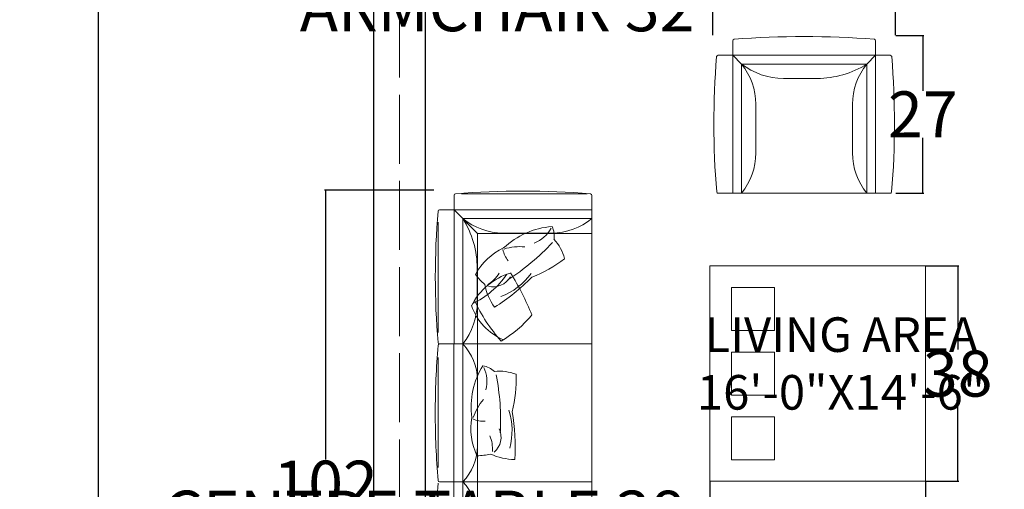
# Model space of a CAD drawing. Units: inches. Extents: x -48 to 50072, y 0 to 21068.
# Tile 49 of 75: x -48 to 123, y 738 to 819. Entities that reach past the tile are written whole.
import ezdxf

# ---------------------------------------------------------------- set-up
doc = ezdxf.new("R2010")
doc.units = ezdxf.units.IN
doc.header["$MEASUREMENT"] = 0
doc.linetypes.add('ACAD_ISO02W100', pattern=[15, 12, -3])
for name, color, linetype, lineweight in [('A-ANNO-DIMS', 2, 'Continuous', 18), ('A-AREA-IDEN', 7, 'Continuous', 18), ('C-PROP', 7, 'Continuous', 25), ('C-PROP-REF', 32, 'ACAD_ISO02W100', 13), ('FURNITURE', 44, 'Continuous', 18)]:
    doc.layers.add(name, color=color, linetype=linetype, lineweight=lineweight)
doc.styles.get("Standard").update_dxf_attribs({"font": 'arial.ttf'})
doc.dimstyles.get("Standard").update_dxf_attribs({"dimtxt": 8, "dimasz": 0.18, "dimexe": 0.18, "dimexo": 0.0625, "dimgap": 0.09, "dimtad": 0, "dimtih": 1, "dimtoh": 1, "dimdec": 1, "dimzin": 0, "dimdsep": 46, "dimlunit": 4, "dimtxsty": 'Standard', "dimblk": 'ARCHTICK', "dimcen": 0.09, "dimadec": 0, "dimazin": 0, "dimtfac": 1, "dimtdec": 1, "dimtofl": 0, "dimtmove": 0, "dimatfit": 3, "dimldrblk": 'ARCHTICK', "dimfxl": 1, "dimtolj": 1, "dimtzin": 0, "dimarcsym": 0})

# ---------------------------------------------------------------- blocks, each defined once
blk = doc.blocks.new('CENTER TABLE')
at = {"layer": 'FURNITURE'}
for points in [[(7434.06, 1871.2), (7464.06, 1871.2), (7464.06, 1901.2), (7434.06, 1901.2)], [(7455.06, 1898.2), (7461.06, 1898.2), (7461.06, 1892.2), (7455.06, 1892.2)], [(7455.06, 1883.2), (7461.06, 1883.2), (7461.06, 1889.2), (7455.06, 1889.2)], [(7455.06, 1874.2), (7461.06, 1874.2), (7461.06, 1880.2), (7455.06, 1880.2)]]:
    blk.add_lwpolyline(points, close=True, dxfattribs=at)
blk = doc.blocks.new('WRG')
at = {"layer": 'FURNITURE'}
for centre, radius, start, end in [((-5881.03, 869.32), 50.97, 111.3371, 122.4176), ((-5914.7, 898.39), 23.82, 30.3068, 50.5663), ((-5895.33, 916.33), 13.61, 197.0126, 242.9429), ((-5918.49, 896.36), 18.43, 25.9005, 55.6513), ((-5905.57, 915.66), 12.15, 289.4501, 336.7699), ((-5915.78, 934.22), 32.17, 294.0815, 312.2768)]:
    blk.add_arc(centre, radius, start, end, dxfattribs=at)
blk = doc.blocks.new('DFGS')
at = {"layer": 'FURNITURE'}
for centre, radius, start, end in [((-6087.14, 813.36), 9.64, 104.9394, 132.5633), ((-6112.38, 805.26), 28.66, 21.6133, 37.4184), ((-6094.33, 816.04), 4.48, 81.3108, 116.3418), ((-6126.91, 783.89), 49.66, 32.8076, 46.9), ((-6080.05, 821.2), 16.31, 184.0297, 223.6176), ((-6099.45, 813.66), 7.12, 22.214, 60.8038), ((-6080.96, 813.35), 11.17, 174.5959, 197.1556), ((-6094.76, 804.41), 13.97, 20.7975, 53.8819), ((-6116.99, 784.16), 44.49, 32.4999, 45.375), ((-6080.21, 815.37), 12.85, 204.9913, 241.6537), ((-6092.61, 815.13), 5.43, 281.6061, 309.1892), ((-6087.9, 807.73), 4.17, 346.5527, 60.4145), ((-6089.91, 803.33), 6.58, 30.5945, 59.6065), ((-6086.56, 817.99), 12.2, 280.9279, 305.5545), ((-6095.16, 815.51), 14.47, 307.7029, 318.9387)]:
    blk.add_arc(centre, radius, start, end, dxfattribs=at)
blk = doc.blocks.new('3+2 seater sofa')
at = {"layer": 'FURNITURE'}
for p, q in [((1464.23, 900.93), (1464.23, 875.06)), ((1465.03, 901.17), (1486.94, 901.17)), ((1488.22, 900.95), (1488.22, 898.4)), ((1488.22, 898.4), (1464.22, 898.4)), ((1488.22, 898.4), (1484.13, 894.31)), ((1490.75, 898.4), (1488.22, 898.4)), ((1488.22, 898.4), (1488.22, 875.06, 0)), ((1486.69, 896.88), (1464.22, 896.88)), ((1486.69, 896.88), (1486.69, 875.06)), ((1490.98, 877.03), (1490.98, 896.27)), ((1484.13, 894.31, 0), (1464.22, 894.31)), ((1471.21, 894.37), (1479.69, 894.37)), ((1484.13, 894.31), (1484.13, 875.06)), ((1484.18, 888.22), (1484.18, 882.36)), ((1490.74, 875.06), (1464.23, 875.06)), ((1484.13, 875.06), (1490.75, 875.06)), ((1486.69, 863.06), (1486.69, 875.06)), ((1488.23, 851.03, 0), (1488.23, 875.06)), ((1490.98, 872.68), (1490.98, 863.06)), ((1484.15, 868.83), (1484.15, 863.06)), ((1484.15, 857.29), (1484.15, 863.06)), ((1484.15, 863.06, 0), (1484.15, 851.06)), ((1486.69, 863.06), (1486.69, 851.06)), ((1490.98, 853.57), (1490.98, 863.06)), ((1490.74, 851.06), (1464.23, 851.06)), ((1484.13, 851.06), (1490.75, 851.06)), ((1486.69, 839.06), (1486.69, 851.06)), ((1488.23, 827.03, 0), (1488.23, 851.06)), ((1490.98, 848.68), (1490.98, 839.06)), ((1484.15, 844.83), (1484.15, 839.06)), ((1484.15, 833.29), (1484.15, 839.06)), ((1484.15, 839.06, 0), (1484.15, 827.06)), ((1486.69, 839.06), (1486.69, 827.06)), ((1490.98, 829.57), (1490.98, 839.06)), ((1366.11, 826.25), (1366.11, 804.34)), ((1366.35, 827.06), (1392.23, 827.06)), ((1368.88, 803.07), (1368.88, 827.07)), ((1370.4, 804.59), (1370.4, 827.07)), ((1392.23, 800.54), (1392.23, 827.06)), ((1392.23, 800.54), (1392.23, 827.06)), ((1416.23, 800.54), (1416.23, 827.06)), ((1440.23, 800.54), (1440.23, 827.06)), ((1464.23, 800.54), (1464.23, 827.06)), ((1490.74, 827.06), (1464.23, 827.06)), ((1484.13, 827.06), (1490.75, 827.06)), ((1372.92, 820.07), (1372.92, 811.59)), ((1368.88, 803.07), (1372.97, 807.16)), ((1372.97, 807.16), (1392.23, 807.16)), ((1379.07, 807.11), (1384.92, 807.11)), ((1392.23, 807.16), (1392.23, 800.53)), ((1392.23, 807.16), (1392.23, 800.53)), ((1398.46, 807.13), (1404.23, 807.13)), ((1410, 807.13), (1404.23, 807.13)), ((1404.23, 807.13, 0), (1416.23, 807.13)), ((1416.23, 807.16), (1416.23, 800.53)), ((1422.46, 807.13), (1428.23, 807.13)), ((1434, 807.13), (1428.23, 807.13)), ((1428.23, 807.13, 0), (1440.23, 807.13)), ((1440.23, 807.16), (1440.23, 800.53)), ((1446.46, 807.13), (1452.23, 807.13)), ((1458, 807.13), (1452.23, 807.13)), ((1452.23, 807.13, 0), (1464.23, 807.13)), ((1464.23, 807.16), (1464.23, 800.53)), ((1370.4, 804.59), (1392.23, 804.59)), ((1404.23, 804.59), (1392.23, 804.59)), ((1404.23, 804.59), (1416.23, 804.59)), ((1428.23, 804.59), (1416.23, 804.59)), ((1428.23, 804.59), (1440.23, 804.59)), ((1452.23, 804.59), (1440.23, 804.59)), ((1452.23, 804.59), (1464.23, 804.59)), ((1366.33, 803.07), (1368.88, 803.07)), ((1368.88, 800.53), (1368.88, 803.07)), ((1368.88, 803.07), (1392.23, 803.07, 0)), ((1416.26, 803.06, 0), (1392.23, 803.06)), ((1440.26, 803.06, 0), (1416.23, 803.06)), ((1464.26, 803.06, 0), (1440.23, 803.06)), ((1390.25, 800.3), (1371.02, 800.3)), ((1394.6, 800.3), (1404.23, 800.3)), ((1413.72, 800.3), (1404.23, 800.3)), ((1418.6, 800.3), (1428.23, 800.3)), ((1437.72, 800.3), (1428.23, 800.3)), ((1442.6, 800.3), (1452.23, 800.3)), ((1461.72, 800.3), (1452.23, 800.3))]:
    blk.add_line(p, q, dxfattribs=at)
at = {"layer": 'FURNITURE', "ltscale": 3}
for p, q in [((1464.23, 875.06), (1464.23, 851.06)), ((1484.15, 863.06), (1484.15, 875.06)), ((1484.15, 863.06), (1484.15, 851.06)), ((1464.23, 851.06), (1464.23, 827.06)), ((1484.15, 839.06), (1484.15, 851.06)), ((1484.15, 839.06), (1484.15, 827.06)), ((1392.23, 827.06), (1416.23, 827.06)), ((1416.23, 827.06), (1440.23, 827.06)), ((1440.23, 827.06), (1464.23, 827.06)), ((1404.23, 807.13), (1392.23, 807.13)), ((1404.23, 807.13), (1416.23, 807.13)), ((1428.23, 807.13), (1416.23, 807.13)), ((1428.23, 807.13), (1440.23, 807.13)), ((1452.23, 807.13), (1440.23, 807.13)), ((1452.23, 807.13), (1464.23, 807.13))]:
    blk.add_line(p, q, dxfattribs=at)
at = {"layer": 'FURNITURE'}
for centre, radius, start, end in [((1476.31, 758.13), 143.55, 85.3368, 94.7395), ((1464.47, 900.93), 0.255, 94.7915, 180), ((1487.96, 900.95), 0.255, 0, 85.2857), ((1490.75, 898.15), 0.255, 5.7807, 90), ((1354.3, 886.73), 137.18, 355.2142, 4.7858), ((1471.31, 905.62), 11.26, 230.9515, 269.5157), ((1479.6, 905.62), 11.26, 270.4843, 309.0485), ((1500.6, 888.15), 16.42, 147.8787, 179.7559), ((1496.3, 882.45), 12.13, 180.424, 217.563), ((1493.43, 868.68), 9.28, 136.5598, 179.0844), ((1490.74, 874.8), 0.255, 4.5067, 90), ((1490.75, 875.31), 0.255, 270, 354.2193), ((1348.3, 862.96), 143.19, 0.0378, 4.7508), ((1348.3, 863.15), 143.19, 355.2492, 359.9622), ((1493.43, 857.43), 9.28, 180.9156, 223.4402), ((1493.43, 844.68), 9.28, 136.5598, 179.0844), ((1490.74, 851.31), 0.255, 270, 355.4933), ((1348.3, 838.96), 143.19, 0.0378, 4.7508), ((1348.3, 839.15), 143.19, 355.2492, 359.9622), ((1493.43, 833.43), 9.28, 180.9156, 223.4402), ((1509.16, 814.97), 143.55, 175.2605, 184.6632), ((1366.35, 826.81), 0.255, 90, 175.2085), ((1361.66, 819.98), 11.26, 0.4843, 39.0485), ((1490.74, 827.31), 0.255, 270, 355.4933), ((1361.66, 811.68), 11.26, 320.9515, 359.5157), ((1379.14, 790.68), 16.42, 90.2441, 122.1213), ((1384.83, 794.98), 12.13, 52.437, 89.576), ((1398.61, 797.86), 9.28, 90.9156, 133.4402), ((1409.85, 797.86), 9.28, 46.5598, 89.0844), ((1422.61, 797.86), 9.28, 90.9156, 133.4402), ((1433.85, 797.86), 9.28, 46.5598, 89.0844), ((1446.61, 797.86), 9.28, 90.9156, 133.4402), ((1457.85, 797.86), 9.28, 46.5598, 89.0844), ((1366.33, 803.32), 0.255, 184.7143, 270), ((1369.13, 800.53), 0.255, 180, 264.2193), ((1380.55, 936.98), 137.18, 265.2142, 274.7858), ((1391.97, 800.54), 0.255, 274.5067, 0), ((1391.97, 800.53), 0.255, 275.7807, 0), ((1392.48, 800.54), 0.255, 180, 265.4933), ((1392.48, 800.53), 0.255, 180, 264.2193), ((1404.32, 942.98), 143.19, 265.2492, 269.9622), ((1404.13, 942.98), 143.19, 270.0378, 274.7508), ((1415.97, 800.54), 0.255, 274.5067, 0), ((1428.32, 942.98), 143.19, 265.2492, 269.9622), ((1428.13, 942.98), 143.19, 270.0378, 274.7508), ((1439.97, 800.54), 0.255, 274.5067, 0), ((1452.32, 942.98), 143.19, 265.2492, 269.9622), ((1452.13, 942.98), 143.19, 270.0378, 274.7508), ((1463.97, 800.54), 0.255, 274.5067, 0)]:
    blk.add_arc(centre, radius, start, end, dxfattribs=at)
at = {"layer": 'FURNITURE', "yscale": 0.8336162403020807, "zscale": 0.8336162403020807}
for name, p, xscale, rotation in [('DFGS', (2154.78, -4186.5, 0), -0.8336162403020807, 90), ('WRG', (2238.95, -4037.88), -0.8336162403020807, 90), ('DFGS', (-2239.7, -2654.91), -0.8336162403020807, 35.78436137719967), ('DFGS', (-2239.7, -2678.91), -0.8336162403020807, 35.78436137719967), ('DFGS', (4922.38, 4530.98), 0.8336162403020807, 54.21563862280032), ('DFGS', (4946.38, 4530.98), 0.8336162403020807, 54.21563862280032), ('DFGS', (4970.38, 4530.98), 0.8336162403020807, 54.21563862280032)]:
    blk.add_blockref(name, p, dxfattribs=dict(at, xscale=xscale, rotation=rotation))
at = {"layer": 'FURNITURE', "xscale": 0.8336162403020807, "yscale": 0.8336162403020807, "zscale": 0.8336162403020807}
for name, p in [('DFGS', (6453.79, 136.5, 0)), ('WRG', (6305.16, 52.33))]:
    blk.add_blockref(name, p, dxfattribs=at)
blk = doc.blocks.new('1 seat sofa')
at = {"layer": 'FURNITURE'}
for p, q in [((1428.81, 918.38), (1428.81, 891.86)), ((1453.69, 918.38), (1453.69, 891.86)), ((1426.27, 915.84), (1456.23, 915.84, 0)), ((1428.81, 915.84), (1430.34, 914.32)), ((1453.69, 915.84), (1452.16, 914.32)), ((1452.16, 914.32), (1430.34, 914.32)), ((1430.34, 914.32), (1430.34, 891.86)), ((1452.16, 914.32), (1452.16, 891.86)), ((1456.26, 891.86), (1426.28, 891.86))]:
    blk.add_line(p, q, dxfattribs=at)
for points in [[(1453.69, 918.38, 0.384962), (1453.46, 918.63, 0.039177), (1429.04, 918.63, 0.384962), (1428.81, 918.38)], [(1426.27, 915.84, 0.390314), (1426.01, 915.61, 0.04105), (1426.03, 892.08, 0.426115), (1426.28, 891.86)], [(1456.23, 915.84, -0.390314), (1456.49, 915.61, -0.04105), (1456.47, 892.08, -0.426115), (1456.22, 891.86)], [(1430.34, 914.32, 0.139995), (1439, 911.81), (1444.86, 911.81, 0.163483), (1452.16, 914.32)], [(1430.34, 891.86, 0.170686), (1432.85, 898.84), (1432.85, 907.32, 0.169875), (1430.34, 914.32)], [(1452.16, 891.86, -0.170686), (1449.65, 898.84), (1449.65, 907.32, -0.169875), (1452.16, 914.32)]]:
    blk.add_lwpolyline(points, format="xyb", dxfattribs=at)
blk = doc.blocks.new('_ArchTick')
at = {"color": 0, "linetype": 'ByBlock', "const_width": 0.15}
blk.add_lwpolyline([(-0.5, -0.5), (0.5, 0.5)], dxfattribs=at)
blk = doc.blocks.new('*D106')
at = {"layer": 'A-ANNO-DIMS', "color": 0, "lineweight": -2, "transparency": 16777216}
for p, q in [((72.04, 738.93), (72.04, 733.18)), ((109.54, 738.93), (109.54, 733.18)), ((72.04, 733.36), (71.86, 733.36)), ((109.54, 733.36), (72.04, 733.36))]:
    blk.add_line(p, q, dxfattribs=at)
at = {"layer": 'Defpoints', "color": 0, "transparency": 16777216}
for p in [(72.04, 738.99), (109.54, 738.99), (72.04, 733.36)]:
    blk.add_point(p, dxfattribs=at)
at = {"layer": 'A-ANNO-DIMS', "color": 0, "lineweight": -2, "transparency": 16777216, "xscale": 0.18, "yscale": 0.18, "zscale": 0.18, "rotation": 180}
blk.add_blockref('_ArchTick', (72.04, 733.36), dxfattribs=at)
at = {"layer": 'A-ANNO-DIMS', "color": 0, "lineweight": -2, "transparency": 16777216, "xscale": 0.18, "yscale": 0.18, "zscale": 0.18}
blk.add_blockref('_ArchTick', (109.54, 733.36), dxfattribs=at)
at = {"layer": 'A-ANNO-DIMS', "color": 0, "transparency": 16777216, "insert": (22.3, 733.36), "char_height": 8, "attachment_point": 5}
blk.add_mtext('\\A1;CENTRE TABLE 38', dxfattribs=at)
blk = doc.blocks.new('*D107')
at = {"layer": 'A-ANNO-DIMS', "color": 0, "lineweight": -2, "transparency": 16777216}
for p, q in [((109.6, 776.49), (115.35, 776.49)), ((115.17, 776.49), (115.17, 761.92)), ((115.17, 738.99), (115.17, 753.56)), ((109.6, 738.99), (115.35, 738.99))]:
    blk.add_line(p, q, dxfattribs=at)
at = {"layer": 'Defpoints', "color": 0, "transparency": 16777216}
for p in [(109.54, 776.49), (109.54, 738.99), (115.17, 738.99)]:
    blk.add_point(p, dxfattribs=at)
at = {"layer": 'A-ANNO-DIMS', "color": 0, "lineweight": -2, "transparency": 16777216, "xscale": 0.18, "yscale": 0.18, "zscale": 0.18}
for p, rotation in [((115.17, 776.49), 90), ((115.17, 738.99), 270)]:
    blk.add_blockref('_ArchTick', p, dxfattribs=dict(at, rotation=rotation))
at = {"layer": 'A-ANNO-DIMS', "color": 0, "transparency": 16777216, "insert": (115.17, 757.74), "char_height": 8, "attachment_point": 5}
blk.add_mtext('\\A1;38', dxfattribs=at)
blk = doc.blocks.new('*D109')
at = {"layer": 'A-ANNO-DIMS', "color": 0, "lineweight": -2, "transparency": 16777216}
for p, q in [((24.03, 789.68), (4.99, 789.68)), ((5.17, 789.68), (5.17, 742.76)), ((5.17, 687.48), (5.17, 734.41)), ((24.03, 687.48), (4.99, 687.48))]:
    blk.add_line(p, q, dxfattribs=at)
at = {"layer": 'Defpoints', "color": 0, "transparency": 16777216}
for p in [(5.17, 789.68), (24.1, 789.68), (24.1, 687.48)]:
    blk.add_point(p, dxfattribs=at)
at = {"layer": 'A-ANNO-DIMS', "color": 0, "lineweight": -2, "transparency": 16777216, "xscale": 0.18, "yscale": 0.18, "zscale": 0.18}
for p, rotation in [((5.17, 789.68), 90), ((5.17, 687.48), 270)]:
    blk.add_blockref('_ArchTick', p, dxfattribs=dict(at, rotation=rotation))
at = {"layer": 'A-ANNO-DIMS', "color": 0, "transparency": 16777216, "insert": (5.17, 738.58), "char_height": 8, "attachment_point": 5}
blk.add_mtext('\\A1;102', dxfattribs=at)
blk = doc.blocks.new('*D110')
at = {"layer": 'A-ANNO-DIMS', "color": 0, "lineweight": -2, "transparency": 16777216}
for p, q in [((72.57, 821.34), (72.39, 821.34)), ((72.57, 816.64), (72.57, 821.52)), ((104.32, 821.34), (72.57, 821.34)), ((104.32, 816.64), (104.32, 821.52))]:
    blk.add_line(p, q, dxfattribs=at)
at = {"layer": 'Defpoints', "color": 0, "transparency": 16777216}
for p in [(72.57, 821.34), (72.57, 816.58), (104.32, 816.58)]:
    blk.add_point(p, dxfattribs=at)
at = {"layer": 'A-ANNO-DIMS', "color": 0, "lineweight": -2, "transparency": 16777216, "xscale": 0.18, "yscale": 0.18, "zscale": 0.18, "rotation": 180}
blk.add_blockref('_ArchTick', (72.57, 821.34), dxfattribs=at)
at = {"layer": 'A-ANNO-DIMS', "color": 0, "lineweight": -2, "transparency": 16777216, "xscale": 0.18, "yscale": 0.18, "zscale": 0.18}
blk.add_blockref('_ArchTick', (104.32, 821.34), dxfattribs=at)
at = {"layer": 'A-ANNO-DIMS', "color": 0, "transparency": 16777216, "insert": (35.02, 821.34), "char_height": 8, "attachment_point": 5}
blk.add_mtext('\\A1;ARMCHAIR 32', dxfattribs=at)
blk = doc.blocks.new('*D111')
at = {"layer": 'A-ANNO-DIMS', "color": 0, "lineweight": -2, "transparency": 16777216}
for p, q in [((104.39, 816.58), (109.27, 816.58)), ((109.09, 816.58), (109.09, 806.98)), ((109.09, 789.16), (109.09, 798.76)), ((104.39, 789.16), (109.27, 789.16))]:
    blk.add_line(p, q, dxfattribs=at)
at = {"layer": 'Defpoints', "color": 0, "transparency": 16777216}
for p in [(104.32, 816.58), (109.09, 816.58), (104.32, 789.16)]:
    blk.add_point(p, dxfattribs=at)
at = {"layer": 'A-ANNO-DIMS', "color": 0, "lineweight": -2, "transparency": 16777216, "xscale": 0.18, "yscale": 0.18, "zscale": 0.18}
for p, rotation in [((109.09, 816.58), 90), ((109.09, 789.16), 270)]:
    blk.add_blockref('_ArchTick', p, dxfattribs=dict(at, rotation=rotation))
at = {"layer": 'A-ANNO-DIMS', "color": 0, "transparency": 16777216, "insert": (109.09, 802.87), "char_height": 8, "attachment_point": 5}
blk.add_mtext('\\A1;27', dxfattribs=at)
blk = doc.blocks.new('*D113')
at = {"layer": 'A-ANNO-DIMS', "color": 0, "lineweight": -2, "transparency": 16777216}
for p, q in [((13.45, 1170.77), (-34.61, 1170.77)), ((-34.43, 1170.77), (-34.43, 696.6)), ((-34.43, 214.07), (-34.43, 688.25)), ((13.45, 214.07), (-34.61, 214.07))]:
    blk.add_line(p, q, dxfattribs=at)
at = {"layer": 'Defpoints', "color": 0, "transparency": 16777216}
for p in [(-34.43, 1170.77), (13.52, 1170.77), (13.52, 214.07)]:
    blk.add_point(p, dxfattribs=at)
at = {"layer": 'A-ANNO-DIMS', "color": 0, "lineweight": -2, "transparency": 16777216, "xscale": 0.18, "yscale": 0.18, "zscale": 0.18}
for p, rotation in [((-34.43, 1170.77), 90), ((-34.43, 214.07), 270)]:
    blk.add_blockref('_ArchTick', p, dxfattribs=dict(at, rotation=rotation))
at = {"layer": 'A-ANNO-DIMS', "color": 0, "transparency": 16777216, "insert": (-34.43, 692.42), "char_height": 8, "attachment_point": 5}
blk.add_mtext('\\A1;956.7', dxfattribs=at)

msp = doc.modelspace()

# ---------------------------------------------------------------- linework, layer by layer
at = {"layer": 'C-PROP'}
for p, q in [((13.517, 1170.775), (13.517, 214.075)), ((22.517, 860.775), (22.517, 223.075))]:
    msp.add_line(p, q, dxfattribs=at)
at = {"layer": 'C-PROP-REF'}
msp.add_line((18.017, 1166.275), (18.017, 214.075), dxfattribs=at)

# ---------------------------------------------------------------- block references
at = {"layer": 'FURNITURE', "xscale": -1}
for name, p in [('1 seat sofa', (1529.697, -102.69)), ('3+2 seater sofa', (1515.738, -112.158))]:
    msp.add_blockref(name, p, dxfattribs=at)
at = {"layer": 'FURNITURE', "xscale": 1.25, "yscale": 1.25, "zscale": 1.25, "rotation": 180}
msp.add_blockref('CENTER TABLE', (9402.122, 3115.492), dxfattribs=at)

# ---------------------------------------------------------------- texts
at = {"layer": 'A-AREA-IDEN', "insert": (16.167, 767.541), "char_height": 6.02726, "attachment_point": 1}
msp.add_mtext_dynamic_manual_height_columns('\\pxqc;LIVING AREA ^J16\'-0"X14\'-6"', width=157.39154, gutter_width=30.136, heights=[0], dxfattribs=at)

# ---------------------------------------------------------------- dimensions: what is measured, and where the dimension line sits
at = {"layer": 'A-ANNO-DIMS'}
for base, p1, p2, angle, override, picture, middle in [((-34.433, 1170.775), (13.517, 214.075), (13.517, 1170.775), 90, {"dimdec": 1, "dimlfac": 1, "dimrnd": 0, "dimzin": 0, "dimdsep": 46, "dimlunit": 2}, '*D113', (-34.433, 692.425)), ((109.085, 816.58), (104.323, 789.161), (104.323, 816.58), 90, {"dimdec": 0, "dimlfac": 1, "dimrnd": 0, "dimzin": 0, "dimdsep": 46, "dimlunit": 2}, '*D111', (109.085, 802.871)), ((5.167, 789.685), (24.097, 687.484), (24.097, 789.685), 90, {"dimdec": 0, "dimlfac": 1, "dimrnd": 0, "dimzin": 0, "dimdsep": 46, "dimlunit": 2}, '*D109', (5.167, 738.584)), ((115.167451158, 738.987887343), (109.542451158, 776.487887343), (109.542451158, 738.987887343), 270, {"dimdec": 0, "dimlfac": 1, "dimrnd": 0, "dimzin": 0, "dimdsep": 46, "dimlunit": 2}, '*D107', (115.167451158, 757.737887343))]:
    dim = msp.add_linear_dim(base=base, p1=p1, p2=p2, angle=angle, dimstyle='Standard', override=override, dxfattribs=at)
    dim.commit()
    dim.dimension.update_dxf_attribs({"geometry": picture, "text_midpoint": middle})
for base, p1, p2, text, picture, middle in [((72.572, 821.343), (104.323, 816.58), (72.572, 816.58), 'ARMCHAIR <>', '*D110', (35.025, 821.343)), ((72.042451158, 733.362887343), (109.542451158, 738.987887343), (72.042451158, 738.987887343), 'CENTRE TABLE <>', '*D106', (22.29905416, 733.362887343))]:
    dim = msp.add_linear_dim(base=base, p1=p1, p2=p2, angle=180, text=text, dimstyle='Standard', override={"dimdec": 0, "dimlfac": 1, "dimrnd": 0, "dimzin": 0, "dimdsep": 46, "dimlunit": 2}, dxfattribs=at)
    dim.commit()
    dim.dimension.update_dxf_attribs({"geometry": picture, "text_midpoint": middle})

doc.saveas('drawing.dxf')
